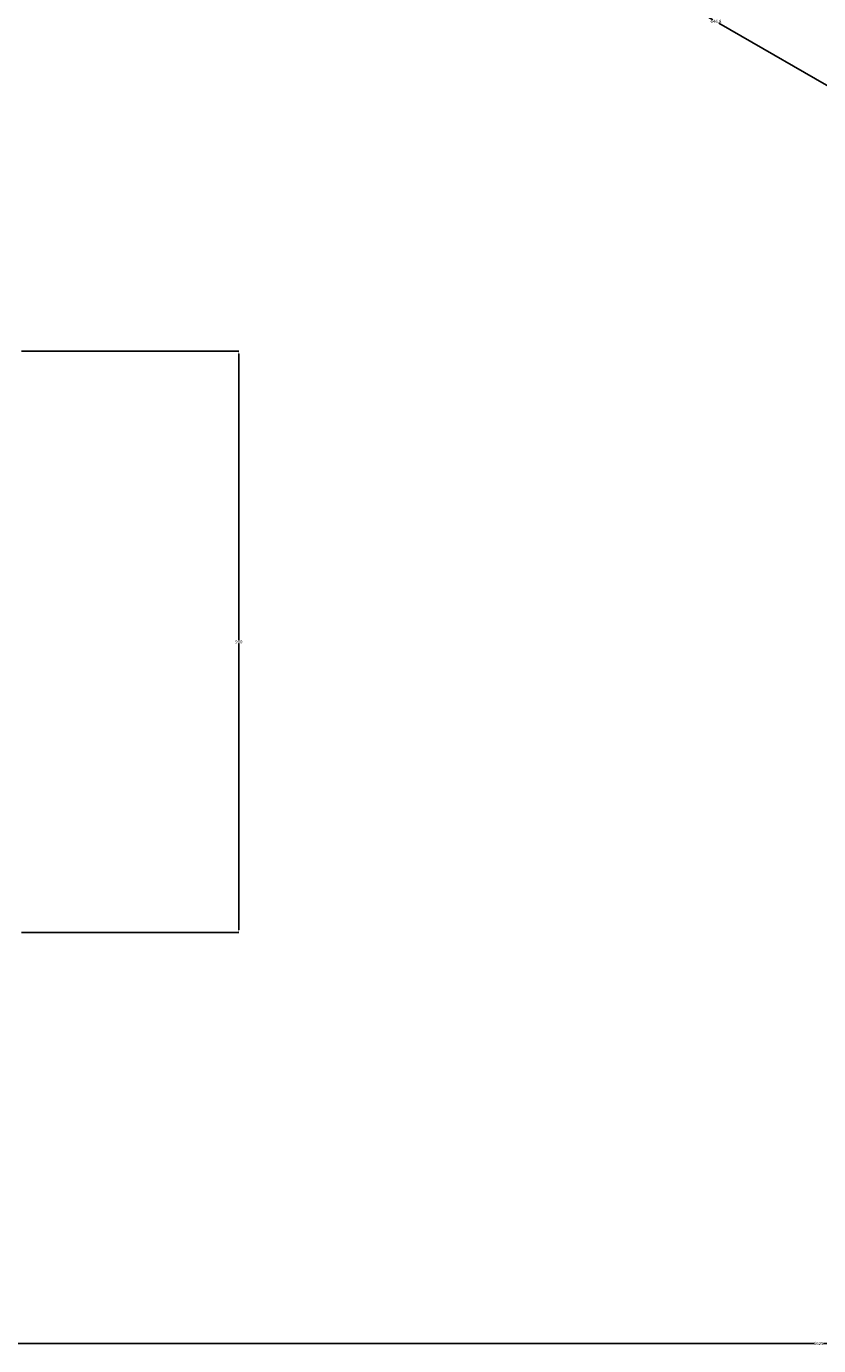
# Model space of a CAD drawing. Units: metres. Extents: x -2391 to 4922, y -635 to 4845.
# Tile 11 of 37: x 39 to 1265, y -635 to 1408. Entities that reach past the tile are written whole.
import ezdxf

# ---------------------------------------------------------------- set-up
doc = ezdxf.new("R2010")
doc.units = ezdxf.units.M
doc.header["$MEASUREMENT"] = 0
doc.layers.add('A-ANNO-DIMS', color=2, linetype='Continuous', lineweight=18)
doc.styles.get("Standard").update_dxf_attribs({"font": 'arial.ttf'})
doc.dimstyles.get("Standard").update_dxf_attribs({"dimtxt": 5, "dimasz": 4, "dimexe": 0.18, "dimexo": 0.0625, "dimgap": 0.09, "dimtad": 0, "dimtih": 1, "dimtoh": 1, "dimdec": 0, "dimzin": 0, "dimdsep": 46, "dimtxsty": 'Standard', "dimcen": 0.09, "dimadec": 0, "dimazin": 0, "dimtfac": 1, "dimtdec": 0, "dimtofl": 0, "dimtmove": 0, "dimatfit": 3, "dimfxl": 1, "dimtolj": 1, "dimtzin": 0, "dimarcsym": 0})

# ---------------------------------------------------------------- blocks, each defined once
blk = doc.blocks.new('*D8')
at = {"layer": 'A-ANNO-DIMS', "color": 0, "lineweight": -2, "transparency": 16777216}
for p, q in [((-2047.3, 3005.2), (-2047.3, -631.4)), ((4577.8, 2350.2), (4577.8, -631.4)), ((-2043.3, -631.2), (1257.6, -631.2)), ((4573.8, -631.2), (1272.8, -631.2))]:
    blk.add_line(p, q, dxfattribs=at)
at = {"layer": 'A-ANNO-DIMS', "color": 0, "transparency": 16777216}
for points in [[(-2043.3, -630.6), (-2043.3, -631.9), (-2047.3, -631.2)], [(4573.8, -630.6), (4573.8, -631.9), (4577.8, -631.2)]]:
    blk.add_solid(points, dxfattribs=at)
at = {"layer": 'Defpoints', "color": 0, "transparency": 16777216}
for p in [(-2047.3, 3005.3), (4577.8, 2350.3), (4577.8, -631.2)]:
    blk.add_point(p, dxfattribs=at)
at = {"layer": 'A-ANNO-DIMS', "color": 0, "transparency": 16777216, "insert": (1265.2, -631.2), "char_height": 5, "attachment_point": 5}
blk.add_mtext('\\A1;6625', dxfattribs=at)
blk = doc.blocks.new('*D10')
at = {"layer": 'A-ANNO-DIMS', "color": 0, "lineweight": -2, "transparency": 16777216}
for p, q in [((550.7, 4505.3), (-2384, 4505.3)), ((-2383.8, 4501.3), (-2383.8, 2107.9)), ((-2383.8, -290.7), (-2383.8, 2102.6)), ((-488.6, -294.7), (-2384, -294.7))]:
    blk.add_line(p, q, dxfattribs=at)
at = {"layer": 'A-ANNO-DIMS', "color": 0, "transparency": 16777216}
for points in [[(-2384.5, 4501.3), (-2383.2, 4501.3), (-2383.8, 4505.3)], [(-2384.5, -290.7), (-2383.2, -290.7), (-2383.8, -294.7)]]:
    blk.add_solid(points, dxfattribs=at)
at = {"layer": 'Defpoints', "color": 0, "transparency": 16777216}
for p in [(-2383.8, 4505.3), (550.7, 4505.3), (-488.5, -294.7)]:
    blk.add_point(p, dxfattribs=at)
at = {"layer": 'A-ANNO-DIMS', "color": 0, "transparency": 16777216, "insert": (-2383.8, 2105.3), "char_height": 5, "attachment_point": 5}
blk.add_mtext('\\A1;4800', dxfattribs=at)
blk = doc.blocks.new('*D19')
at = {"layer": 'A-ANNO-DIMS', "color": 0, "lineweight": -2, "transparency": 16777216}
for p, q in [((994.5, 1869), (826.2, 1577.5)), ((829.7, 1575.6), (1101.7, 1418.6)), ((1554.6, 1545.6), (1386.3, 1254.1)), ((1382.9, 1256.3), (1110.9, 1413.3))]:
    blk.add_line(p, q, dxfattribs=at)
at = {"layer": 'A-ANNO-DIMS', "color": 0, "transparency": 16777216}
for points in [[(830.1, 1576.2), (829.4, 1575.1), (826.3, 1577.6)], [(1383.2, 1256.8), (1382.6, 1255.7), (1386.4, 1254.3)]]:
    blk.add_solid(points, dxfattribs=at)
at = {"layer": 'Defpoints', "color": 0, "transparency": 16777216}
for p in [(994.5, 1869.1), (826.3, 1577.6), (1554.6, 1545.7)]:
    blk.add_point(p, dxfattribs=at)
at = {"layer": 'A-ANNO-DIMS', "color": 0, "transparency": 16777216, "insert": (1106.3, 1416), "char_height": 5, "attachment_point": 5}
blk.add_mtext('\\A1;646.8', dxfattribs=at)
blk = doc.blocks.new('*D48')
at = {"layer": 'A-ANNO-DIMS', "color": 0, "lineweight": -2, "transparency": 16777216}
for p, q in [((31.2, 905.3), (367.8, 905.3)), ((367.6, 901.3), (367.6, 457.9)), ((367.6, 9.3), (367.6, 452.6)), ((31.2, 5.3), (367.8, 5.3))]:
    blk.add_line(p, q, dxfattribs=at)
at = {"layer": 'A-ANNO-DIMS', "color": 0, "transparency": 16777216}
for points in [[(367, 901.3), (368.3, 901.3), (367.6, 905.3)], [(367, 9.3), (368.3, 9.3), (367.6, 5.3)]]:
    blk.add_solid(points, dxfattribs=at)
at = {"layer": 'Defpoints', "color": 0, "transparency": 16777216}
for p in [(31.1, 905.3), (31.1, 5.3), (367.6, 5.3)]:
    blk.add_point(p, dxfattribs=at)
at = {"layer": 'A-ANNO-DIMS', "color": 0, "transparency": 16777216, "insert": (367.6, 455.3), "char_height": 5, "attachment_point": 5}
blk.add_mtext('\\A1;900', dxfattribs=at)

msp = doc.modelspace()

# ---------------------------------------------------------------- dimensions: what is measured, and where the dimension line sits
at = {"layer": 'A-ANNO-DIMS'}
for base, p1, p2, angle, override, picture, middle in [((-2383.8343, 4505.2763), (-488.4886, -294.7237), (550.7419, 4505.2763), 90, {"dimdec": 0, "dimlfac": 1, "dimrnd": 0, "dimzin": 0, "dimdsep": 46, "dimlunit": 2}, '*D10', (-2383.8343, 2105.2763)), ((826.2603, 1577.6489), (1554.6155, 1545.6896), (994.5103, 1869.0664), 150, {"dimdec": 1, "dimlfac": 1, "dimrnd": 0, "dimzin": 0, "dimdsep": 46, "dimlunit": 2}, '*D19', (1106.3129, 1415.9604)), ((367.6266, 5.2763), (31.1266, 905.2763), (31.1266, 5.2763), 270, {"dimdec": 0, "dimlfac": 1, "dimrnd": 0, "dimzin": 0, "dimdsep": 46, "dimlunit": 2}, '*D48', (367.6266, 455.2763))]:
    dim = msp.add_linear_dim(base=base, p1=p1, p2=p2, angle=angle, dimstyle='Standard', override=override, dxfattribs=at)
    dim.commit()
    dim.dimension.update_dxf_attribs({"geometry": picture, "text_midpoint": middle})
dim = msp.add_linear_dim(base=(4577.76, -631.2237), p1=(-2047.3343, 3005.2763), p2=(4577.76, 2350.2763), dimstyle='Standard', override={"dimdec": 0, "dimlfac": 1, "dimrnd": 0, "dimzin": 0, "dimdsep": 46, "dimlunit": 2}, dxfattribs=at)
dim.commit()
dim.dimension.update_dxf_attribs({"geometry": '*D8', "text_midpoint": (1265.2128, -631.2237)})

doc.saveas('drawing.dxf')
